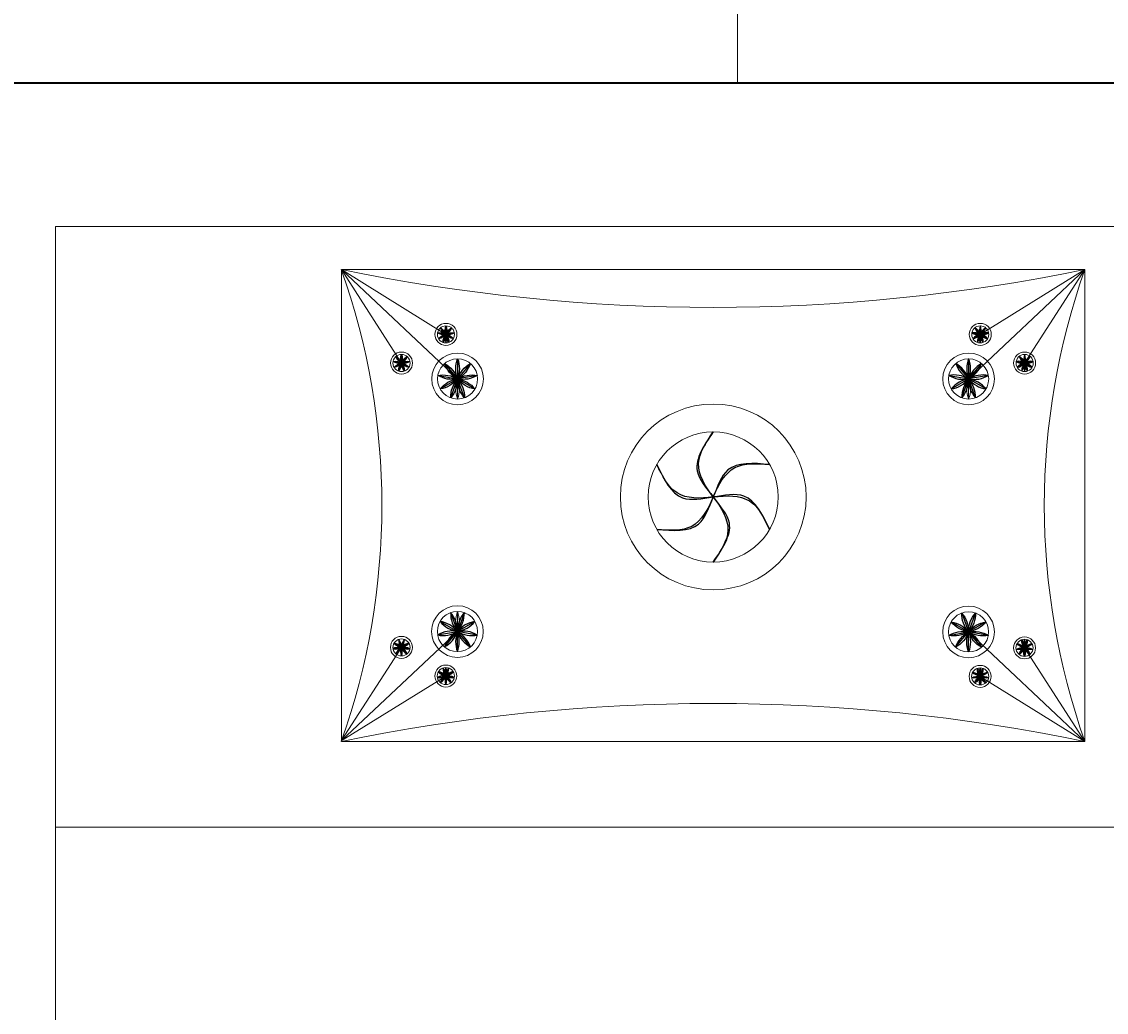
# Model space of a CAD drawing. Units: inches. Extents: x -46 to 1145, y -527 to 760.
# Tile 39 of 57: x 53 to 83, y 625 to 652. Entities that reach past the tile are written whole.
import ezdxf

# ---------------------------------------------------------------- set-up
doc = ezdxf.new("R2010")
doc.units = ezdxf.units.IN
doc.header["$MEASUREMENT"] = 0
for name, color, linetype, lineweight in [('A-ANNO-DIMS', 2, 'Continuous', 18), ('A-FURN', 2, 'Continuous', 13), ('WALLS', 4, 'Continuous', 40), ('WINDOWS', 240, 'Continuous', 20)]:
    doc.layers.add(name, color=color, linetype=linetype, lineweight=lineweight)
doc.layers.add('FURNTIURE', color=2, linetype='Continuous')
doc.layers.add('LT', color=9, linetype='Continuous')
doc.styles.get("Standard").update_dxf_attribs({"font": 'arial.ttf'})
doc.dimstyles.get("Standard").update_dxf_attribs({"dimtxt": 0.18, "dimasz": 0.18, "dimexe": 0.18, "dimexo": 0.0625, "dimgap": 0.09, "dimtad": 0, "dimtih": 1, "dimtoh": 1, "dimdec": 0, "dimzin": 0, "dimdsep": 46, "dimlunit": 3, "dimtxsty": 'Standard', "dimcen": 0.09, "dimadec": 0, "dimazin": 0, "dimtfac": 1, "dimtdec": 0, "dimtofl": 0, "dimtmove": 0, "dimatfit": 3, "dimfxl": 1, "dimtolj": 1, "dimtzin": 0, "dimarcsym": 0})

# ---------------------------------------------------------------- blocks, each defined once
blk = doc.blocks.new('WINDOW-36IN')
blk.add_line((0, 9), (0, 0))
blk = doc.blocks.new('*U34')
at = {"layer": 'LT'}
blk.add_line((0, 0.281), (0, -0.281), dxfattribs=at)
for centre, start, end in [((0.734, 0), 159.0676, 200.9324), ((-0.734, 0), 339.0676, 20.9324)]:
    blk.add_arc(centre, 0.786, start, end, dxfattribs=at)
blk = doc.blocks.new('*U35')
at = {"layer": 'LT', "transparency": 16777216}
for p, rotation in [((609.756, 443.96), 40.00000000000002), ((610.117, 443.96), 320), ((609.659, 443.794), 80.00000000000001), ((609.693, 443.605), 120), ((609.84, 443.481), 160), ((610.032, 443.481), 200), ((610.179, 443.605), 240), ((610.213, 443.794), 280)]:
    blk.add_blockref('*U34', p, dxfattribs=dict(at, rotation=rotation))
blk.add_blockref('*U34', (609.936, 444.026), dxfattribs=at)
blk = doc.blocks.new('*U36')
at = {"layer": 'LT'}
blk.add_line((0, 0.12), (0, -0.12), dxfattribs=at)
for centre, start, end in [((0.313, 0), 159.0676, 200.9324), ((-0.313, 0), 339.0676, 20.9324)]:
    blk.add_arc(centre, 0.335, start, end, dxfattribs=at)
blk = doc.blocks.new('*U37')
at = {"layer": 'LT', "transparency": 16777216}
for p, rotation in [((259.536, 188.967), 40), ((259.69, 188.967), 320), ((259.495, 188.896), 80.00000000000001), ((259.509, 188.816), 120), ((259.572, 188.763), 160), ((259.654, 188.763), 200), ((259.716, 188.816), 240), ((259.731, 188.896), 280)]:
    blk.add_blockref('*U36', p, dxfattribs=dict(at, rotation=rotation))
blk.add_blockref('*U36', (259.613, 188.995), dxfattribs=at)
blk = doc.blocks.new('*U38')
at = {"layer": 'LT'}
blk.add_line((0, 0.12), (0, -0.12), dxfattribs=at)
for centre, start, end in [((0.313, 0), 159.0676, 200.9324), ((-0.313, 0), 339.0676, 20.9324)]:
    blk.add_arc(centre, 0.335, start, end, dxfattribs=at)
blk = doc.blocks.new('*U39')
at = {"layer": 'LT', "transparency": 16777216}
for p, rotation in [((259.536, 188.967), 40), ((259.69, 188.967), 320), ((259.495, 188.896), 80.00000000000001), ((259.509, 188.816), 120), ((259.572, 188.763), 160), ((259.654, 188.763), 200), ((259.716, 188.816), 240), ((259.731, 188.896), 280)]:
    blk.add_blockref('*U38', p, dxfattribs=dict(at, rotation=rotation))
blk.add_blockref('*U38', (259.613, 188.995), dxfattribs=at)
blk = doc.blocks.new('*U40')
at = {"layer": 'LT'}
blk.add_line((0, 0.281), (0, -0.281), dxfattribs=at)
for centre, start, end in [((0.734, 0), 159.0676, 200.9324), ((-0.734, 0), 339.0676, 20.9324)]:
    blk.add_arc(centre, 0.786, start, end, dxfattribs=at)
blk = doc.blocks.new('*U41')
at = {"layer": 'LT', "transparency": 16777216}
for p, rotation in [((609.756, 443.96), 40.00000000000002), ((610.117, 443.96), 320), ((609.659, 443.794), 80.00000000000001), ((609.693, 443.605), 120), ((609.84, 443.481), 160), ((610.032, 443.481), 200), ((610.179, 443.605), 240), ((610.213, 443.794), 280)]:
    blk.add_blockref('*U40', p, dxfattribs=dict(at, rotation=rotation))
blk.add_blockref('*U40', (609.936, 444.026), dxfattribs=at)
blk = doc.blocks.new('*U42')
at = {"layer": 'LT'}
blk.add_line((0, 0.12), (0, -0.12), dxfattribs=at)
for centre, start, end in [((0.313, 0), 159.0676, 200.9324), ((-0.313, 0), 339.0676, 20.9324)]:
    blk.add_arc(centre, 0.335, start, end, dxfattribs=at)
blk = doc.blocks.new('*U43')
at = {"layer": 'LT', "transparency": 16777216}
for p, rotation in [((259.536, 188.967), 40), ((259.69, 188.967), 320), ((259.495, 188.896), 80.00000000000001), ((259.509, 188.816), 120), ((259.572, 188.763), 160), ((259.654, 188.763), 200), ((259.716, 188.816), 240), ((259.731, 188.896), 280)]:
    blk.add_blockref('*U42', p, dxfattribs=dict(at, rotation=rotation))
blk.add_blockref('*U42', (259.613, 188.995), dxfattribs=at)
blk = doc.blocks.new('*U44')
at = {"layer": 'LT'}
blk.add_line((0, 0.12), (0, -0.12), dxfattribs=at)
for centre, start, end in [((0.313, 0), 159.0676, 200.9324), ((-0.313, 0), 339.0676, 20.9324)]:
    blk.add_arc(centre, 0.335, start, end, dxfattribs=at)
blk = doc.blocks.new('*U45')
at = {"layer": 'LT', "transparency": 16777216}
for p, rotation in [((259.536, 188.967), 40), ((259.69, 188.967), 320), ((259.495, 188.896), 80.00000000000001), ((259.509, 188.816), 120), ((259.572, 188.763), 160), ((259.654, 188.763), 200), ((259.716, 188.816), 240), ((259.731, 188.896), 280)]:
    blk.add_blockref('*U44', p, dxfattribs=dict(at, rotation=rotation))
blk.add_blockref('*U44', (259.613, 188.995), dxfattribs=at)
blk = doc.blocks.new('*U72')
at = {"layer": 'LT'}
blk.add_line((0, 0.281), (0, -0.281), dxfattribs=at)
for centre, start, end in [((0.734, 0), 159.0676, 200.9324), ((-0.734, 0), 339.0676, 20.9324)]:
    blk.add_arc(centre, 0.786, start, end, dxfattribs=at)
blk = doc.blocks.new('*U73')
at = {"layer": 'LT', "transparency": 16777216}
for p, rotation in [((609.756, 443.96), 40.00000000000002), ((610.117, 443.96), 320), ((609.659, 443.794), 80.00000000000001), ((609.693, 443.605), 120), ((609.84, 443.481), 160), ((610.032, 443.481), 200), ((610.179, 443.605), 240), ((610.213, 443.794), 280)]:
    blk.add_blockref('*U72', p, dxfattribs=dict(at, rotation=rotation))
blk.add_blockref('*U72', (609.936, 444.026), dxfattribs=at)
blk = doc.blocks.new('*U74')
at = {"layer": 'LT'}
blk.add_line((0, 0.12), (0, -0.12), dxfattribs=at)
for centre, start, end in [((0.313, 0), 159.0676, 200.9324), ((-0.313, 0), 339.0676, 20.9324)]:
    blk.add_arc(centre, 0.335, start, end, dxfattribs=at)
blk = doc.blocks.new('*U75')
at = {"layer": 'LT', "transparency": 16777216}
for p, rotation in [((259.536, 188.967), 40), ((259.69, 188.967), 320), ((259.495, 188.896), 80.00000000000001), ((259.509, 188.816), 120), ((259.572, 188.763), 160), ((259.654, 188.763), 200), ((259.716, 188.816), 240), ((259.731, 188.896), 280)]:
    blk.add_blockref('*U74', p, dxfattribs=dict(at, rotation=rotation))
blk.add_blockref('*U74', (259.613, 188.995), dxfattribs=at)
blk = doc.blocks.new('*U76')
at = {"layer": 'LT'}
blk.add_line((0, 0.12), (0, -0.12), dxfattribs=at)
for centre, start, end in [((0.313, 0), 159.0676, 200.9324), ((-0.313, 0), 339.0676, 20.9324)]:
    blk.add_arc(centre, 0.335, start, end, dxfattribs=at)
blk = doc.blocks.new('*U77')
at = {"layer": 'LT', "transparency": 16777216}
for p, rotation in [((259.536, 188.967), 40), ((259.69, 188.967), 320), ((259.495, 188.896), 80.00000000000001), ((259.509, 188.816), 120), ((259.572, 188.763), 160), ((259.654, 188.763), 200), ((259.716, 188.816), 240), ((259.731, 188.896), 280)]:
    blk.add_blockref('*U76', p, dxfattribs=dict(at, rotation=rotation))
blk.add_blockref('*U76', (259.613, 188.995), dxfattribs=at)
blk = doc.blocks.new('*U78')
at = {"layer": 'LT'}
blk.add_line((0, 0.281), (0, -0.281), dxfattribs=at)
for centre, start, end in [((0.734, 0), 159.0676, 200.9324), ((-0.734, 0), 339.0676, 20.9324)]:
    blk.add_arc(centre, 0.786, start, end, dxfattribs=at)
blk = doc.blocks.new('*U79')
at = {"layer": 'LT', "transparency": 16777216}
for p, rotation in [((609.756, 443.96), 40.00000000000002), ((610.117, 443.96), 320), ((609.659, 443.794), 80.00000000000001), ((609.693, 443.605), 120), ((609.84, 443.481), 160), ((610.032, 443.481), 200), ((610.179, 443.605), 240), ((610.213, 443.794), 280)]:
    blk.add_blockref('*U78', p, dxfattribs=dict(at, rotation=rotation))
blk.add_blockref('*U78', (609.936, 444.026), dxfattribs=at)
blk = doc.blocks.new('*U80')
at = {"layer": 'LT'}
blk.add_line((0, 0.12), (0, -0.12), dxfattribs=at)
for centre, start, end in [((0.313, 0), 159.0676, 200.9324), ((-0.313, 0), 339.0676, 20.9324)]:
    blk.add_arc(centre, 0.335, start, end, dxfattribs=at)
blk = doc.blocks.new('*U81')
at = {"layer": 'LT', "transparency": 16777216}
for p, rotation in [((259.536, 188.967), 40), ((259.69, 188.967), 320), ((259.495, 188.896), 80.00000000000001), ((259.509, 188.816), 120), ((259.572, 188.763), 160), ((259.654, 188.763), 200), ((259.716, 188.816), 240), ((259.731, 188.896), 280)]:
    blk.add_blockref('*U80', p, dxfattribs=dict(at, rotation=rotation))
blk.add_blockref('*U80', (259.613, 188.995), dxfattribs=at)
blk = doc.blocks.new('*U82')
at = {"layer": 'LT'}
blk.add_line((0, 0.12), (0, -0.12), dxfattribs=at)
for centre, start, end in [((0.313, 0), 159.0676, 200.9324), ((-0.313, 0), 339.0676, 20.9324)]:
    blk.add_arc(centre, 0.335, start, end, dxfattribs=at)
blk = doc.blocks.new('*U83')
at = {"layer": 'LT', "transparency": 16777216}
for p, rotation in [((259.536, 188.967), 40), ((259.69, 188.967), 320), ((259.495, 188.896), 80.00000000000001), ((259.509, 188.816), 120), ((259.572, 188.763), 160), ((259.654, 188.763), 200), ((259.716, 188.816), 240), ((259.731, 188.896), 280)]:
    blk.add_blockref('*U82', p, dxfattribs=dict(at, rotation=rotation))
blk.add_blockref('*U82', (259.613, 188.995), dxfattribs=at)
blk = doc.blocks.new('*U32')
at = {"layer": 'FURNTIURE'}
blk.add_open_spline([(0.039, 1.82), (-0.218, 1.447), (-0.661, 0.801), (0.102, -0.025), (0.645, -0.928), (0.238, -1.527), (0.039, -1.82)], degree=3, knots=[0, 0, 0, 0, 1.177175, 2.037162, 3.056205, 4.032246, 4.032246, 4.032246, 4.032246], dxfattribs=at)
blk = doc.blocks.new('*U33')
at = {"layer": 'FURNTIURE', "transparency": 16777216}
blk.add_blockref('*U32', (904.302, 663.383), dxfattribs=at)
for p, rotation in [((904.379, 663.383), 180), ((904.321, 663.416), 300), ((904.321, 663.349), 59.99999999999999), ((904.36, 663.416), 239.9999999999999), ((904.36, 663.349), 119.9999999999999)]:
    blk.add_blockref('*U32', p, dxfattribs=dict(at, rotation=rotation))
blk = doc.blocks.new('BED-QUEEN-FURNISHED')
for p, q in [((0, 0), (0, 80)), ((0, 80), (60, 80)), ((8, 78.8), (28.8, 78.8)), ((8, 65.6), (8, 78.8)), ((8, 78.8), (11.385, 75.613)), ((8, 78.8), (9.684, 76.184)), ((8, 78.8), (10.926, 76.984)), ((28.8, 78.8), (25.415, 75.613)), ((28.8, 78.8), (25.874, 76.984)), ((28.8, 78.8), (27.115, 76.184)), ((28.8, 78.8), (28.8, 65.6)), ((10.926, 76.984), (10.926, 76.745)), ((25.874, 76.984), (25.874, 76.745)), ((27.115, 76.184), (27.115, 75.945)), ((11.251, 75.739), (11.251, 75.177)), ((25.548, 75.739), (25.548, 75.177)), ((11.249, 68.673), (11.249, 69.235)), ((7.995, 65.614), (11.382, 68.799)), ((28.795, 65.6), (25.412, 68.789)), ((27.112, 68.216), (27.113, 68.456)), ((7.995, 65.614), (9.682, 68.228)), ((28.795, 65.6), (27.112, 68.216)), ((10.923, 67.428), (10.923, 67.667)), ((7.995, 65.614), (10.923, 67.428)), ((25.87, 67.418), (25.87, 67.657)), ((28.795, 65.6), (25.87, 67.418)), ((8, 65.6), (28.8, 65.6)), ((60, 63.2), (0, 63.2))]:
    blk.add_line(p, q)
for centre, radius in [((10.926, 76.984), 0.308), ((10.926, 76.984), 0.239), ((25.874, 76.984), 0.308), ((25.874, 76.984), 0.239), ((9.684, 76.184), 0.308), ((11.251, 75.739), 0.723), ((25.548, 75.739), 0.723), ((27.115, 76.184), 0.308), ((9.684, 76.184), 0.239), ((11.251, 75.739), 0.562), ((25.548, 75.739), 0.562), ((27.115, 76.184), 0.239), ((18.404, 72.437), 2.599), ((18.404, 72.437), 1.82), ((11.249, 68.673), 0.723), ((11.249, 68.673), 0.562), ((25.546, 68.663), 0.723), ((25.546, 68.663), 0.562), ((9.682, 68.228), 0.308), ((9.682, 68.228), 0.239), ((27.112, 68.216), 0.308), ((27.112, 68.216), 0.239), ((10.923, 67.428), 0.308), ((10.923, 67.428), 0.239), ((25.87, 67.418), 0.308), ((25.87, 67.418), 0.239)]:
    blk.add_circle(centre, radius)
for centre, radius, start, end in [((18.4, 129.177), 51.439, 258.3356, 281.6644), ((-10.654, 72.2), 19.787, 340.5151, 19.4849), ((47.453, 72.2), 19.787, 160.5151, 199.4849), ((11.239, 76.865), 0.335, 159.0676, 200.9324), ((10.614, 76.865), 0.335, 339.0676, 20.9324), ((26.186, 76.865), 0.335, 159.0676, 200.9324), ((25.561, 76.865), 0.335, 339.0676, 20.9324), ((27.428, 76.065), 0.335, 159.0676, 200.9324), ((26.803, 76.065), 0.335, 339.0676, 20.9324), ((11.985, 75.458), 0.786, 159.0676, 200.9324), ((10.517, 75.458), 0.786, 339.0676, 20.9324), ((26.283, 75.458), 0.786, 159.0676, 200.9324), ((24.814, 75.458), 0.786, 339.0676, 20.9324), ((11.983, 68.953), 0.786, 159.028, 200.8928), ((10.515, 68.954), 0.786, 339.028, 20.8928), ((27.425, 68.336), 0.335, 159.028, 200.8928), ((26.8, 68.336), 0.335, 339.028, 20.8928), ((11.235, 67.547), 0.335, 159.028, 200.8928), ((10.61, 67.548), 0.335, 339.028, 20.8928), ((26.183, 67.537), 0.335, 159.028, 200.8928), ((25.558, 67.537), 0.335, 339.028, 20.8928), ((18.4, 15.223), 51.439, 78.3356, 101.6644)]:
    blk.add_arc(centre, radius, start, end)
at = {"xscale": -1}
for name, p in [('*U45', (270.539, -111.891)), ('*U43', (269.297, -112.691)), ('*U41', (621.187, -368.006))]:
    blk.add_blockref(name, p, dxfattribs=at)
for name, p in [('*U39', (-233.739, -111.891)), ('*U35', (-584.388, -368.006)), ('*U37', (-232.498, -112.691)), ('*U33', (-885.936, -590.946))]:
    blk.add_blockref(name, p)
at = {"rotation": 179.9603994254766}
for name, p in [('*U79', (621.491, 511.997)), ('*U81', (269.425, 256.925)), ('*U83', (270.666, 256.124))]:
    blk.add_blockref(name, p, dxfattribs=at)
at = {"xscale": -1, "rotation": 179.9603994254766}
for name, p in [('*U73', (-584.083, 512.83)), ('*U75', (-232.37, 257.271)), ('*U77', (-233.612, 256.472))]:
    blk.add_blockref(name, p, dxfattribs=at)
blk = doc.blocks.new('*D685')
at = {"layer": 'A-ANNO-DIMS', "color": 0, "lineweight": -2, "transparency": 16777216}
for p, q in [((183.501, 700.889), (-46.216, 700.889)), ((-46.036, 700.709), (-46.036, 116.385)), ((-46.036, -468.302), (-46.036, 116.021)), ((12.501, -468.482), (-46.216, -468.482))]:
    blk.add_line(p, q, dxfattribs=at)
at = {"layer": 'A-ANNO-DIMS', "color": 0, "transparency": 16777216}
for points in [[(-46.066, 700.709), (-46.006, 700.709), (-46.036, 700.889)], [(-46.066, -468.302), (-46.006, -468.302), (-46.036, -468.482)]]:
    blk.add_solid(points, dxfattribs=at)
at = {"layer": 'Defpoints', "color": 0, "transparency": 16777216}
for p in [(-46.036, 700.889), (183.564, 700.889), (12.564, -468.482)]:
    blk.add_point(p, dxfattribs=at)
at = {"layer": 'A-ANNO-DIMS', "color": 0, "transparency": 16777216, "insert": (-46.036, 116.203), "char_height": 0.18, "attachment_point": 5}
blk.add_mtext('\\A1;1169.4', dxfattribs=at)

msp = doc.modelspace()

# ---------------------------------------------------------------- linework, layer by layer
at = {"layer": 'WALLS'}
msp.add_line((183.5637, 650.5176), (21.5637, 650.5176), dxfattribs=at)

# ---------------------------------------------------------------- block references
at = {"layer": 'A-FURN'}
msp.add_blockref('BED-QUEEN-FURNISHED', (53.91, 566.503), dxfattribs=at)
at = {"layer": 'WINDOWS'}
msp.add_blockref('WINDOW-36IN', (72.995, 650.518), dxfattribs=at)

# ---------------------------------------------------------------- dimensions: what is measured, and where the dimension line sits
at = {"layer": 'A-ANNO-DIMS'}
dim = msp.add_linear_dim(base=(-46.0363, 700.8886), p1=(12.5637, -468.4824), p2=(183.5637, 700.8886), angle=90, dimstyle='Standard', override={"dimdec": 1, "dimlfac": 1, "dimrnd": 0, "dimzin": 0, "dimdsep": 46, "dimlunit": 2}, dxfattribs=at)
dim.commit()
dim.dimension.update_dxf_attribs({"geometry": '*D685', "text_midpoint": (-46.0363, 116.2031)})

doc.saveas('drawing.dxf')
